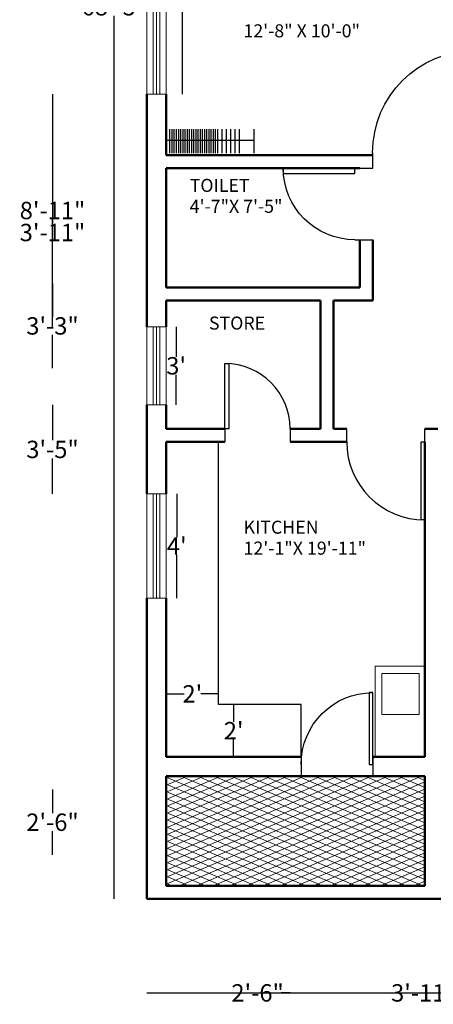
# Model space of a CAD drawing. Units: inches. Extents: x -135167 to -134597, y 156853 to 157819.
# Tile 1 of 5: x -135161 to -134971, y 156853 to 157306. Entities that reach past the tile are written whole.
import ezdxf

# ---------------------------------------------------------------- set-up
doc = ezdxf.new("R2010")
doc.units = ezdxf.units.IN
doc.header["$MEASUREMENT"] = 0
for name, color, linetype, lineweight in [('A-ANNO-DIMS', 4, 'Continuous', 18), ('A-AREA-IDEN', 76, 'Continuous', 25), ('A-FLOR-CASE', 1, 'Continuous', 25), ('A-FLOR-FIXT', 3, 'Continuous', 20), ('A-FLOR-PATT', 8, 'Continuous', 13), ('doors', 5, 'Continuous', 25), ('walls', 2, 'Continuous', 50), ('window', 6, 'Continuous', 18)]:
    doc.layers.add(name, color=color, linetype=linetype, lineweight=lineweight)
doc.styles.get("Standard").update_dxf_attribs({"font": 'arial.ttf'})
doc.dimstyles.get("Standard").update_dxf_attribs({"dimtxt": 8, "dimasz": 0.18, "dimexe": 0.18, "dimexo": 0.0625, "dimgap": 0.09, "dimtad": 0, "dimtih": 1, "dimtoh": 1, "dimdec": 0, "dimzin": 0, "dimdsep": 46, "dimlunit": 3, "dimtxsty": 'Standard', "dimblk": 'ARCHTICK', "dimcen": 0.09, "dimse1": 1, "dimse2": 1, "dimadec": 0, "dimazin": 0, "dimtfac": 1, "dimtdec": 0, "dimtofl": 0, "dimtmove": 0, "dimatfit": 3, "dimldrblk": 'DOTSMALL', "dimfxl": 1, "dimtolj": 1, "dimtzin": 0, "dimarcsym": 0})

# ---------------------------------------------------------------- blocks, each defined once
blk = doc.blocks.new('*U13')
for p, q in [((0, 0), (0, -6)), ((30, 0), (30, -6))]:
    blk.add_line(p, q)
blk.add_lwpolyline([(0, 0), (0, 30), (1.75, 30), (1.75, 0)], close=True)
blk.add_arc((0, 0), 30, 0, 90)
blk = doc.blocks.new('*U6')
for p, q in [((0, 0), (0, -6)), ((40, 0), (40, -6))]:
    blk.add_line(p, q)
blk.add_lwpolyline([(0, 0), (0, 40), (1.75, 40), (1.75, 0)], close=True)
blk.add_arc((0, 0), 40, 0, 90)
blk = doc.blocks.new('*U12')
for p, q in [((0, 0), (0, -6)), ((24, 0), (24, -6))]:
    blk.add_line(p, q)
blk.add_lwpolyline([(0, 0), (0, 24), (1.75, 24), (1.75, 0)], close=True)
blk.add_arc((0, 0), 24, 0, 90)
blk = doc.blocks.new('*U14')
for p, q in [((0, 0), (0, -6)), ((36, 0), (36, -6))]:
    blk.add_line(p, q)
blk.add_lwpolyline([(0, 0), (0, 36), (1.75, 36), (1.75, 0)], close=True)
blk.add_arc((0, 0), 36, 0, 90)
blk = doc.blocks.new('*U9')
for p, q in [((-36, 0), (-36, 6)), ((0, 0), (0, 6))]:
    blk.add_line(p, q)
blk.add_lwpolyline([(0, 0), (0, -36), (-1.75, -36), (-1.75, 0)], close=True)
blk.add_arc((0, 0), 36, 180, 270)
blk = doc.blocks.new('_ArchTick')
at = {"color": 0, "linetype": 'ByBlock', "const_width": 0.15}
blk.add_lwpolyline([(-0.5, -0.5), (0.5, 0.5)], dxfattribs=at)
blk = doc.blocks.new('*D20')
at = {"layer": 'A-ANNO-DIMS', "color": 0, "lineweight": -2, "transparency": 16777216}
for p, q in [((-135117.79, 157722.94), (-135117.79, 157316.42)), ((-135117.79, 156901.55), (-135117.79, 157308.07))]:
    blk.add_line(p, q, dxfattribs=at)
at = {"layer": 'Defpoints', "color": 0, "transparency": 16777216}
for p in [(-135117.79, 157722.94), (-135102.89, 157722.94), (-135102.89, 156901.55)]:
    blk.add_point(p, dxfattribs=at)
at = {"layer": 'A-ANNO-DIMS', "color": 0, "lineweight": -2, "transparency": 16777216, "xscale": 0.18, "yscale": 0.18, "zscale": 0.18}
for p, rotation in [((-135117.79, 157722.94), 90), ((-135117.79, 156901.55), 270)]:
    blk.add_blockref('_ArchTick', p, dxfattribs=dict(at, rotation=rotation))
at = {"layer": 'A-ANNO-DIMS', "color": 0, "transparency": 16777216, "insert": (-135117.79, 157312.25), "char_height": 8, "attachment_point": 5}
blk.add_mtext('\\A1;68\'-5"', dxfattribs=at)
blk = doc.blocks.new('_DotSmall')
at = {"color": 0, "linetype": 'ByBlock', "const_width": 0.5}
blk.add_lwpolyline([(-0.0625, 0, 1), (0.0625, 0, 1)], format="xyb", close=True, dxfattribs=at)
blk = doc.blocks.new('*D33')
at = {"layer": 'A-ANNO-DIMS', "color": 0, "lineweight": -2, "transparency": 16777216}
for p, q in [((-135086.43, 157367.94), (-135086.43, 157324.12)), ((-135086.43, 157271.94), (-135086.43, 157315.77))]:
    blk.add_line(p, q, dxfattribs=at)
at = {"layer": 'Defpoints', "color": 0, "transparency": 16777216}
for p in [(-135093.89, 157367.94), (-135086.43, 157367.94), (-135093.89, 157271.94)]:
    blk.add_point(p, dxfattribs=at)
at = {"layer": 'A-ANNO-DIMS', "color": 0, "lineweight": -2, "transparency": 16777216, "xscale": 0.18, "yscale": 0.18, "zscale": 0.18}
for p, rotation in [((-135086.43, 157367.94), 90), ((-135086.43, 157271.94), 270)]:
    blk.add_blockref('_ArchTick', p, dxfattribs=dict(at, rotation=rotation))
at = {"layer": 'A-ANNO-DIMS', "color": 0, "transparency": 16777216, "insert": (-135086.43, 157319.94), "char_height": 8, "attachment_point": 5}
blk.add_mtext("\\A1;8'", dxfattribs=at)
blk = doc.blocks.new('*D34')
at = {"layer": 'A-ANNO-DIMS', "color": 0, "lineweight": -2, "transparency": 16777216}
for p, q in [((-135089.35, 157164.94), (-135089.35, 157151.12)), ((-135089.35, 157128.94), (-135089.35, 157142.77))]:
    blk.add_line(p, q, dxfattribs=at)
at = {"layer": 'Defpoints', "color": 0, "transparency": 16777216}
for p in [(-135093.89, 157164.94), (-135089.35, 157164.94), (-135093.89, 157128.94)]:
    blk.add_point(p, dxfattribs=at)
at = {"layer": 'A-ANNO-DIMS', "color": 0, "lineweight": -2, "transparency": 16777216, "xscale": 0.18, "yscale": 0.18, "zscale": 0.18}
for p, rotation in [((-135089.35, 157164.94), 90), ((-135089.35, 157128.94), 270)]:
    blk.add_blockref('_ArchTick', p, dxfattribs=dict(at, rotation=rotation))
at = {"layer": 'A-ANNO-DIMS', "color": 0, "transparency": 16777216, "insert": (-135089.35, 157146.94), "char_height": 8, "attachment_point": 5}
blk.add_mtext("\\A1;3'", dxfattribs=at)
blk = doc.blocks.new('*D35')
at = {"layer": 'A-ANNO-DIMS', "color": 0, "lineweight": -2, "transparency": 16777216}
for p, q in [((-135089.08, 157087.94), (-135089.08, 157068.03)), ((-135089.08, 157039.94), (-135089.08, 157059.85))]:
    blk.add_line(p, q, dxfattribs=at)
at = {"layer": 'Defpoints', "color": 0, "transparency": 16777216}
for p in [(-135093.89, 157087.94), (-135089.08, 157087.94), (-135093.89, 157039.94)]:
    blk.add_point(p, dxfattribs=at)
at = {"layer": 'A-ANNO-DIMS', "color": 0, "lineweight": -2, "transparency": 16777216, "xscale": 0.18, "yscale": 0.18, "zscale": 0.18}
for p, rotation in [((-135089.08, 157087.94), 90), ((-135089.08, 157039.94), 270)]:
    blk.add_blockref('_ArchTick', p, dxfattribs=dict(at, rotation=rotation))
at = {"layer": 'A-ANNO-DIMS', "color": 0, "transparency": 16777216, "insert": (-135089.08, 157063.94), "char_height": 8, "attachment_point": 5}
blk.add_mtext("\\A1;4'", dxfattribs=at)
blk = doc.blocks.new('*D36')
at = {"layer": 'A-ANNO-DIMS', "color": 0, "lineweight": -2, "transparency": 16777216}
for p, q in [((-135062.9, 156990.94), (-135062.9, 156983.05)), ((-135062.9, 156966.94), (-135062.9, 156974.84))]:
    blk.add_line(p, q, dxfattribs=at)
at = {"layer": 'Defpoints', "color": 0, "transparency": 16777216}
for p in [(-135060.63, 156990.94), (-135062.9, 156966.94), (-135061.48, 156966.94)]:
    blk.add_point(p, dxfattribs=at)
at = {"layer": 'A-ANNO-DIMS', "color": 0, "lineweight": -2, "transparency": 16777216, "xscale": 0.18, "yscale": 0.18, "zscale": 0.18}
for p, rotation in [((-135062.9, 156990.94), 90), ((-135062.9, 156966.94), 270)]:
    blk.add_blockref('_ArchTick', p, dxfattribs=dict(at, rotation=rotation))
at = {"layer": 'A-ANNO-DIMS', "color": 0, "transparency": 16777216, "insert": (-135062.9, 156978.94), "char_height": 8, "attachment_point": 5}
blk.add_mtext("\\A1;2'", dxfattribs=at)
blk = doc.blocks.new('*D37')
at = {"layer": 'A-ANNO-DIMS', "color": 0, "lineweight": -2, "transparency": 16777216}
for p, q in [((-135093.89, 156995.88), (-135085.72, 156995.88)), ((-135069.89, 156995.88), (-135078.05, 156995.88))]:
    blk.add_line(p, q, dxfattribs=at)
at = {"layer": 'Defpoints', "color": 0, "transparency": 16777216}
for p in [(-135093.89, 156995.88), (-135093.89, 156990.94), (-135069.89, 156990.94)]:
    blk.add_point(p, dxfattribs=at)
at = {"layer": 'A-ANNO-DIMS', "color": 0, "lineweight": -2, "transparency": 16777216, "xscale": 0.18, "yscale": 0.18, "zscale": 0.18, "rotation": 180}
blk.add_blockref('_ArchTick', (-135093.89, 156995.88), dxfattribs=at)
at = {"layer": 'A-ANNO-DIMS', "color": 0, "lineweight": -2, "transparency": 16777216, "xscale": 0.18, "yscale": 0.18, "zscale": 0.18}
blk.add_blockref('_ArchTick', (-135069.89, 156995.88), dxfattribs=at)
at = {"layer": 'A-ANNO-DIMS', "color": 0, "transparency": 16777216, "insert": (-135081.89, 156995.88), "char_height": 8, "attachment_point": 5}
blk.add_mtext("\\A1;2'", dxfattribs=at)
blk = doc.blocks.new('WIN-36IN')
for p, q in [((0, 0), (0, 9)), ((0, 9), (36, 9)), ((0, 6), (36, 6)), ((36, 0), (36, 9)), ((0, 4.5), (36, 4.5)), ((0, 3), (36, 3)), ((0, 0), (36, 0))]:
    blk.add_line(p, q)
blk = doc.blocks.new('WIN-96IN')
for p, q in [((0, 96), (9, 96)), ((0, 96), (0, 0)), ((3, 96), (3, 0)), ((4.5, 96), (4.5, 0)), ((6, 96), (6, 0)), ((9, 96), (9, 0)), ((0, 0), (9, 0))]:
    blk.add_line(p, q)
blk = doc.blocks.new('WIN-48IN')
for p, q in [((0, 48), (9, 48)), ((0, 0), (0, 48)), ((3, 0), (3, 48)), ((4.5, 0), (4.5, 48)), ((6, 0), (6, 48)), ((9, 0), (9, 48)), ((0, 0), (9, 0))]:
    blk.add_line(p, q)
blk = doc.blocks.new('*D54')
at = {"layer": 'A-ANNO-DIMS', "color": 0, "lineweight": -2, "transparency": 16777216}
for p, q in [((-135102.89, 156858.2), (-134897.21, 156858.2)), ((-134663.89, 156858.2), (-134869.56, 156858.2))]:
    blk.add_line(p, q, dxfattribs=at)
at = {"layer": 'Defpoints', "color": 0, "transparency": 16777216}
for p in [(-134663.89, 157136.8), (-135102.89, 156901.55), (-134663.89, 156858.2)]:
    blk.add_point(p, dxfattribs=at)
at = {"layer": 'A-ANNO-DIMS', "color": 0, "lineweight": -2, "transparency": 16777216, "xscale": 0.18, "yscale": 0.18, "zscale": 0.18, "rotation": 180}
blk.add_blockref('_ArchTick', (-135102.89, 156858.2), dxfattribs=at)
at = {"layer": 'A-ANNO-DIMS', "color": 0, "lineweight": -2, "transparency": 16777216, "xscale": 0.18, "yscale": 0.18, "zscale": 0.18}
blk.add_blockref('_ArchTick', (-134663.89, 156858.2), dxfattribs=at)
at = {"layer": 'A-ANNO-DIMS', "color": 0, "transparency": 16777216, "insert": (-134883.39, 156858.2), "char_height": 8, "attachment_point": 5}
blk.add_mtext('\\A1;36\'-7"', dxfattribs=at)
blk = doc.blocks.new('*D59')
at = {"layer": 'A-ANNO-DIMS', "color": 0, "lineweight": -2, "transparency": 16777216}
for p, q in [((-135146.24, 157271.94), (-135146.24, 157222.62)), ((-135146.24, 157164.94), (-135146.24, 157214.27))]:
    blk.add_line(p, q, dxfattribs=at)
at = {"layer": 'Defpoints', "color": 0, "transparency": 16777216}
for p in [(-135102.89, 157271.94), (-135146.24, 157164.94), (-135102.89, 157164.94)]:
    blk.add_point(p, dxfattribs=at)
at = {"layer": 'A-ANNO-DIMS', "color": 0, "lineweight": -2, "transparency": 16777216, "xscale": 0.18, "yscale": 0.18, "zscale": 0.18}
for p, rotation in [((-135146.24, 157271.94), 90), ((-135146.24, 157164.94), 270)]:
    blk.add_blockref('_ArchTick', p, dxfattribs=dict(at, rotation=rotation))
at = {"layer": 'A-ANNO-DIMS', "color": 0, "transparency": 16777216, "insert": (-135146.24, 157218.44), "char_height": 8, "attachment_point": 5}
blk.add_mtext('\\A1;8\'-11"', dxfattribs=at)
blk = doc.blocks.new('*D60')
at = {"layer": 'A-ANNO-DIMS', "color": 0, "lineweight": -2, "transparency": 16777216}
for p, q in [((-135146.24, 157128.94), (-135146.24, 157112.62)), ((-135146.24, 157087.94), (-135146.24, 157104.27))]:
    blk.add_line(p, q, dxfattribs=at)
at = {"layer": 'Defpoints', "color": 0, "transparency": 16777216}
for p in [(-135102.89, 157128.94), (-135146.24, 157087.94), (-135102.89, 157087.94)]:
    blk.add_point(p, dxfattribs=at)
at = {"layer": 'A-ANNO-DIMS', "color": 0, "lineweight": -2, "transparency": 16777216, "xscale": 0.18, "yscale": 0.18, "zscale": 0.18}
for p, rotation in [((-135146.24, 157128.94), 90), ((-135146.24, 157087.94), 270)]:
    blk.add_blockref('_ArchTick', p, dxfattribs=dict(at, rotation=rotation))
at = {"layer": 'A-ANNO-DIMS', "color": 0, "transparency": 16777216, "insert": (-135146.24, 157108.44), "char_height": 8, "attachment_point": 5}
blk.add_mtext('\\A1;3\'-5"', dxfattribs=at)
blk = doc.blocks.new('*D79')
at = {"layer": 'A-ANNO-DIMS', "color": 0, "lineweight": -2, "transparency": 16777216}
for p, q in [((-135146.24, 157231.8), (-135146.24, 157212.48)), ((-135146.24, 157184.8), (-135146.24, 157204.12))]:
    blk.add_line(p, q, dxfattribs=at)
at = {"layer": 'Defpoints', "color": 0, "transparency": 16777216}
for p in [(-135146.24, 157231.8), (-134753.89, 157231.8), (-134753.89, 157184.8)]:
    blk.add_point(p, dxfattribs=at)
at = {"layer": 'A-ANNO-DIMS', "color": 0, "lineweight": -2, "transparency": 16777216, "xscale": 0.18, "yscale": 0.18, "zscale": 0.18}
for p, rotation in [((-135146.24, 157231.8), 90), ((-135146.24, 157184.8), 270)]:
    blk.add_blockref('_ArchTick', p, dxfattribs=dict(at, rotation=rotation))
at = {"layer": 'A-ANNO-DIMS', "color": 0, "transparency": 16777216, "insert": (-135146.24, 157208.3), "char_height": 8, "attachment_point": 5}
blk.add_mtext('\\A1;3\'-11"', dxfattribs=at)
blk = doc.blocks.new('*D80')
at = {"layer": 'A-ANNO-DIMS', "color": 0, "lineweight": -2, "transparency": 16777216}
for p, q in [((-135146.24, 157184.8), (-135146.24, 157169.48)), ((-135146.24, 157145.8), (-135146.24, 157161.12))]:
    blk.add_line(p, q, dxfattribs=at)
at = {"layer": 'Defpoints', "color": 0, "transparency": 16777216}
for p in [(-135146.24, 157184.8), (-134753.89, 157184.8), (-134753.89, 157145.8)]:
    blk.add_point(p, dxfattribs=at)
at = {"layer": 'A-ANNO-DIMS', "color": 0, "lineweight": -2, "transparency": 16777216, "xscale": 0.18, "yscale": 0.18, "zscale": 0.18}
for p, rotation in [((-135146.24, 157184.8), 90), ((-135146.24, 157145.8), 270)]:
    blk.add_blockref('_ArchTick', p, dxfattribs=dict(at, rotation=rotation))
at = {"layer": 'A-ANNO-DIMS', "color": 0, "transparency": 16777216, "insert": (-135146.24, 157165.3), "char_height": 8, "attachment_point": 5}
blk.add_mtext('\\A1;3\'-3"', dxfattribs=at)
blk = doc.blocks.new('*D84')
at = {"layer": 'A-ANNO-DIMS', "color": 0, "lineweight": -2, "transparency": 16777216}
for p, q in [((-134998.89, 156858.2), (-134989.21, 156858.2)), ((-134951.89, 156858.2), (-134961.56, 156858.2))]:
    blk.add_line(p, q, dxfattribs=at)
at = {"layer": 'Defpoints', "color": 0, "transparency": 16777216}
for p in [(-134998.89, 157237.94), (-134951.89, 157237.94), (-134951.89, 156858.2)]:
    blk.add_point(p, dxfattribs=at)
at = {"layer": 'A-ANNO-DIMS', "color": 0, "lineweight": -2, "transparency": 16777216, "xscale": 0.18, "yscale": 0.18, "zscale": 0.18, "rotation": 180}
blk.add_blockref('_ArchTick', (-134998.89, 156858.2), dxfattribs=at)
at = {"layer": 'A-ANNO-DIMS', "color": 0, "lineweight": -2, "transparency": 16777216, "xscale": 0.18, "yscale": 0.18, "zscale": 0.18}
blk.add_blockref('_ArchTick', (-134951.89, 156858.2), dxfattribs=at)
at = {"layer": 'A-ANNO-DIMS', "color": 0, "transparency": 16777216, "insert": (-134975.39, 156858.2), "char_height": 8, "attachment_point": 5}
blk.add_mtext('\\A1;3\'-11"', dxfattribs=at)
blk = doc.blocks.new('*D85')
at = {"layer": 'A-ANNO-DIMS', "color": 0, "lineweight": -2, "transparency": 16777216}
for p, q in [((-134620.54, 157237.94), (-134620.54, 157225.62)), ((-134620.54, 157204.94), (-134620.54, 157217.27))]:
    blk.add_line(p, q, dxfattribs=at)
at = {"layer": 'Defpoints', "color": 0, "transparency": 16777216}
for p in [(-135004.89, 157237.94), (-135004.89, 157204.94), (-134620.54, 157204.94)]:
    blk.add_point(p, dxfattribs=at)
at = {"layer": 'A-ANNO-DIMS', "color": 0, "lineweight": -2, "transparency": 16777216, "xscale": 0.18, "yscale": 0.18, "zscale": 0.18}
for p, rotation in [((-134620.54, 157237.94), 90), ((-134620.54, 157204.94), 270)]:
    blk.add_blockref('_ArchTick', p, dxfattribs=dict(at, rotation=rotation))
at = {"layer": 'A-ANNO-DIMS', "color": 0, "transparency": 16777216, "insert": (-134620.54, 157221.44), "char_height": 8, "attachment_point": 5}
blk.add_mtext('\\A1;2\'-9"', dxfattribs=at)
blk = doc.blocks.new('*D86')
at = {"layer": 'A-ANNO-DIMS', "color": 0, "lineweight": -2, "transparency": 16777216}
for p, q in [((-135010.89, 157806.8), (-135003.61, 157806.8)), ((-134974.89, 157806.8), (-134982.17, 157806.8))]:
    blk.add_line(p, q, dxfattribs=at)
at = {"layer": 'Defpoints', "color": 0, "transparency": 16777216}
for p in [(-134974.89, 157806.8), (-135010.89, 157117.94), (-134974.89, 157117.94)]:
    blk.add_point(p, dxfattribs=at)
at = {"layer": 'A-ANNO-DIMS', "color": 0, "lineweight": -2, "transparency": 16777216, "xscale": 0.18, "yscale": 0.18, "zscale": 0.18, "rotation": 180}
blk.add_blockref('_ArchTick', (-135010.89, 157806.8), dxfattribs=at)
at = {"layer": 'A-ANNO-DIMS', "color": 0, "lineweight": -2, "transparency": 16777216, "xscale": 0.18, "yscale": 0.18, "zscale": 0.18}
blk.add_blockref('_ArchTick', (-134974.89, 157806.8), dxfattribs=at)
at = {"layer": 'A-ANNO-DIMS', "color": 0, "transparency": 16777216, "insert": (-134992.89, 157806.8), "char_height": 8, "attachment_point": 5}
blk.add_mtext('\\A1;3\'-0"', dxfattribs=at)
blk = doc.blocks.new('*D87')
at = {"layer": 'A-ANNO-DIMS', "color": 0, "lineweight": -2, "transparency": 16777216}
for p, q in [((-135066.89, 156858.2), (-135062.68, 156858.2)), ((-135036.89, 156858.2), (-135041.09, 156858.2))]:
    blk.add_line(p, q, dxfattribs=at)
at = {"layer": 'Defpoints', "color": 0, "transparency": 16777216}
for p in [(-135066.89, 157111.94), (-135036.89, 157111.94), (-135036.89, 156858.2)]:
    blk.add_point(p, dxfattribs=at)
at = {"layer": 'A-ANNO-DIMS', "color": 0, "lineweight": -2, "transparency": 16777216, "xscale": 0.18, "yscale": 0.18, "zscale": 0.18, "rotation": 180}
blk.add_blockref('_ArchTick', (-135066.89, 156858.2), dxfattribs=at)
at = {"layer": 'A-ANNO-DIMS', "color": 0, "lineweight": -2, "transparency": 16777216, "xscale": 0.18, "yscale": 0.18, "zscale": 0.18}
blk.add_blockref('_ArchTick', (-135036.89, 156858.2), dxfattribs=at)
at = {"layer": 'A-ANNO-DIMS', "color": 0, "transparency": 16777216, "insert": (-135051.89, 156858.2), "char_height": 8, "attachment_point": 5}
blk.add_mtext('\\A1;2\'-6"', dxfattribs=at)
blk = doc.blocks.new('*D88')
at = {"layer": 'A-ANNO-DIMS', "color": 0, "lineweight": -2, "transparency": 16777216}
for p, q in [((-135031.89, 157806.8), (-135026.18, 157806.8)), ((-134998.89, 157806.8), (-135004.59, 157806.8))]:
    blk.add_line(p, q, dxfattribs=at)
at = {"layer": 'Defpoints', "color": 0, "transparency": 16777216}
for p in [(-134998.89, 157806.8), (-135031.89, 156966.94), (-134998.89, 156966.94)]:
    blk.add_point(p, dxfattribs=at)
at = {"layer": 'A-ANNO-DIMS', "color": 0, "lineweight": -2, "transparency": 16777216, "xscale": 0.18, "yscale": 0.18, "zscale": 0.18, "rotation": 180}
blk.add_blockref('_ArchTick', (-135031.89, 157806.8), dxfattribs=at)
at = {"layer": 'A-ANNO-DIMS', "color": 0, "lineweight": -2, "transparency": 16777216, "xscale": 0.18, "yscale": 0.18, "zscale": 0.18}
blk.add_blockref('_ArchTick', (-134998.89, 157806.8), dxfattribs=at)
at = {"layer": 'A-ANNO-DIMS', "color": 0, "transparency": 16777216, "insert": (-135015.39, 157806.8), "char_height": 8, "attachment_point": 5}
blk.add_mtext('\\A1;2\'-9"', dxfattribs=at)
blk = doc.blocks.new('*D91')
at = {"layer": 'A-ANNO-DIMS', "color": 0, "lineweight": -2, "transparency": 16777216}
for p, q in [((-135146.24, 156951.78), (-135146.24, 156940.95)), ((-135146.24, 156921.78), (-135146.24, 156932.6))]:
    blk.add_line(p, q, dxfattribs=at)
at = {"layer": 'Defpoints', "color": 0, "transparency": 16777216}
for p in [(-134797.39, 156951.78), (-135146.24, 156921.78), (-134797.39, 156921.78)]:
    blk.add_point(p, dxfattribs=at)
at = {"layer": 'A-ANNO-DIMS', "color": 0, "lineweight": -2, "transparency": 16777216, "xscale": 0.18, "yscale": 0.18, "zscale": 0.18}
for p, rotation in [((-135146.24, 156951.78), 90), ((-135146.24, 156921.78), 270)]:
    blk.add_blockref('_ArchTick', p, dxfattribs=dict(at, rotation=rotation))
at = {"layer": 'A-ANNO-DIMS', "color": 0, "transparency": 16777216, "insert": (-135146.24, 156936.78), "char_height": 8, "attachment_point": 5}
blk.add_mtext('\\A1;2\'-6"', dxfattribs=at)
blk = doc.blocks.new('*D92')
at = {"layer": 'A-ANNO-DIMS', "color": 0, "lineweight": -2, "transparency": 16777216}
for p, q in [((-134987.89, 156858.2), (-134955.58, 156858.2)), ((-134901.89, 156858.2), (-134934.2, 156858.2))]:
    blk.add_line(p, q, dxfattribs=at)
at = {"layer": 'Defpoints', "color": 0, "transparency": 16777216}
for p in [(-134987.89, 157647.94), (-134901.89, 157647.94), (-134901.89, 156858.2)]:
    blk.add_point(p, dxfattribs=at)
at = {"layer": 'A-ANNO-DIMS', "color": 0, "lineweight": -2, "transparency": 16777216, "xscale": 0.18, "yscale": 0.18, "zscale": 0.18, "rotation": 180}
blk.add_blockref('_ArchTick', (-134987.89, 156858.2), dxfattribs=at)
at = {"layer": 'A-ANNO-DIMS', "color": 0, "lineweight": -2, "transparency": 16777216, "xscale": 0.18, "yscale": 0.18, "zscale": 0.18}
blk.add_blockref('_ArchTick', (-134901.89, 156858.2), dxfattribs=at)
at = {"layer": 'A-ANNO-DIMS', "color": 0, "transparency": 16777216, "insert": (-134944.89, 156858.2), "char_height": 8, "attachment_point": 5}
blk.add_mtext('\\A1;7\'-2"', dxfattribs=at)

msp = doc.modelspace()

# ---------------------------------------------------------------- hatches: boundary and pattern name
at = {"layer": 'A-FLOR-PATT'}
h = msp.add_hatch(dxfattribs=at)
h.set_pattern_fill('ANSI31', color=256, scale=24, angle=-22.049143, style=0)
h.paths.add_polyline_path([(-135093.89, 156907.55), (-134974.89, 156907.55), (-134974.89, 156957.94), (-135093.89, 156957.94)])
h = msp.add_hatch(dxfattribs=at)
h.set_pattern_fill('ANSI31', color=256, scale=24, angle=112.049143, style=0)
h.paths.add_polyline_path([(-135093.89, 156907.55), (-134974.89, 156907.55), (-134974.89, 156957.94), (-135093.89, 156957.94)])

# ---------------------------------------------------------------- linework, layer by layer
at = {"layer": 'A-FLOR-CASE'}
for p, q in [((-135092.34, 157255.95), (-135092.34, 157244.82)), ((-135091.34, 157255.95), (-135091.34, 157244.82)), ((-135090.34, 157255.95), (-135090.34, 157244.82)), ((-135089.34, 157255.95), (-135089.34, 157244.82)), ((-135088.34, 157255.95), (-135088.34, 157244.82)), ((-135087.34, 157255.95), (-135087.34, 157244.82)), ((-135086.34, 157255.95), (-135086.34, 157244.82)), ((-135085.34, 157255.95), (-135085.34, 157244.82)), ((-135084.34, 157255.95), (-135084.34, 157244.82)), ((-135083.34, 157255.95), (-135083.34, 157244.82)), ((-135082.34, 157255.95), (-135082.34, 157244.82)), ((-135081.34, 157255.95), (-135081.34, 157244.82)), ((-135080.34, 157255.95), (-135080.34, 157244.82)), ((-135079.34, 157255.95), (-135079.34, 157244.82)), ((-135078.34, 157255.95), (-135078.34, 157244.82)), ((-135077.34, 157255.95), (-135077.34, 157244.82)), ((-135076.34, 157255.95), (-135076.34, 157244.82)), ((-135075.34, 157255.95), (-135075.34, 157244.82)), ((-135074.34, 157255.95), (-135074.34, 157244.82)), ((-135073.34, 157255.95), (-135073.34, 157244.82)), ((-135072.34, 157255.95), (-135072.34, 157244.82)), ((-135071.34, 157255.95), (-135071.34, 157244.82)), ((-135070.34, 157255.95), (-135070.34, 157244.82)), ((-135068.34, 157255.95), (-135068.34, 157244.82)), ((-135066.34, 157255.95), (-135066.34, 157244.82)), ((-135064.34, 157255.95), (-135064.34, 157244.82)), ((-135062.34, 157255.95), (-135062.34, 157244.82)), ((-135062.34, 157255.95), (-135062.34, 157244.82)), ((-135060.34, 157255.95), (-135060.34, 157244.82)), ((-135053.65, 157255.95), (-135053.65, 157244.82)), ((-135053.65, 157250.6), (-135093.89, 157250.6)), ((-135069.89, 156990.94), (-135069.89, 157111.94)), ((-135031.89, 156990.94), (-135069.89, 156990.94)), ((-135031.89, 156966.94), (-135031.89, 156990.94))]:
    msp.add_line(p, q, dxfattribs=at)
at = {"layer": 'A-FLOR-FIXT'}
for points in [[(-134974.89, 156966.94), (-134997.84, 156966.94), (-134997.84, 157008.71), (-134974.89, 157008.71)], [(-134994.65, 157005.23), (-134977.54, 157005.23), (-134977.54, 156986.41), (-134994.65, 156986.41)]]:
    msp.add_lwpolyline(points, close=True, dxfattribs=at)
at = {"layer": 'doors'}
for p, q in [((-134998.89, 157237.94), (-134998.89, 157243.94)), ((-135004.89, 157237.94), (-134998.89, 157237.94)), ((-135004.89, 157204.94), (-134998.89, 157204.94)), ((-135066.89, 157117.94), (-135066.89, 157111.94)), ((-135036.89, 157117.94), (-135036.89, 157111.94)), ((-135010.89, 157111.94), (-135010.89, 157117.94)), ((-134974.89, 157111.94), (-134974.89, 157117.94)), ((-135031.89, 156966.94), (-135031.89, 156957.94)), ((-134998.89, 156966.94), (-134998.89, 156957.94))]:
    msp.add_line(p, q, dxfattribs=at)
at = {"layer": 'walls'}
for p, q in [((-135102.89, 157164.94), (-135102.89, 157271.94)), ((-135093.89, 157243.94), (-135093.89, 157271.94)), ((-135093.89, 157243.94), (-134998.89, 157243.94)), ((-135093.89, 157237.94), (-135004.89, 157237.94)), ((-135093.89, 157182.94), (-135093.89, 157237.94)), ((-135004.89, 157182.94), (-135004.89, 157204.94)), ((-134998.89, 157176.94), (-134998.89, 157204.94)), ((-135093.89, 157182.94), (-135004.89, 157182.94)), ((-135093.89, 157176.94), (-135022.89, 157176.94)), ((-135093.89, 157164.94), (-135093.89, 157176.94)), ((-135022.89, 157117.94), (-135022.89, 157176.94)), ((-135016.89, 157117.94), (-135016.89, 157176.94)), ((-135016.89, 157176.94), (-134998.89, 157176.94)), ((-135102.89, 157087.94), (-135102.89, 157128.94)), ((-135093.89, 157117.94), (-135093.89, 157128.94)), ((-135093.89, 157117.94), (-135066.89, 157117.94)), ((-135036.89, 157117.94), (-135022.89, 157117.94)), ((-135016.89, 157117.94), (-135010.89, 157117.94)), ((-134974.89, 157117.94), (-134968.89, 157117.94)), ((-135093.89, 157111.94), (-135066.89, 157111.94)), ((-135093.89, 157087.94), (-135093.89, 157111.94)), ((-135036.89, 157111.94), (-135010.89, 157111.94)), ((-134974.89, 156966.94), (-134974.89, 157111.94)), ((-135102.89, 156901.55), (-135102.89, 157039.94)), ((-135093.89, 156966.94), (-135093.89, 157039.94)), ((-135093.89, 156966.94), (-135031.89, 156966.94)), ((-134998.89, 156966.94), (-134974.89, 156966.94)), ((-135093.89, 156907.55), (-135093.89, 156957.94)), ((-135093.89, 156957.94), (-134998.89, 156957.94)), ((-134998.89, 156957.94), (-134974.89, 156957.94)), ((-134974.89, 156907.55), (-134974.89, 156957.94)), ((-135093.89, 156907.55), (-134974.89, 156907.55)), ((-135102.89, 156901.55), (-134744.89, 156901.55))]:
    msp.add_line(p, q, dxfattribs=at)

# ---------------------------------------------------------------- block references
at = {"layer": 'doors'}
for name, p, xscale, yscale, zscale in [('*U6', (-134951.89, 157245.01), -1.177072109473595, 1.177072109473595, 1.177072109473595), ('*U14', (-134998.89, 156963.44), -0.9168796826214972, 0.9168796826214972, 0.9168796826214972)]:
    msp.add_blockref(name, p, dxfattribs=dict(at, xscale=xscale, yscale=yscale, zscale=zscale))
at = {"layer": 'doors', "xscale": -1.373377664918856, "yscale": 1.373377664918856, "zscale": 1.373377664918856, "rotation": 90}
msp.add_blockref('*U12', (-135007.1, 157237.94), dxfattribs=at)
at = {"layer": 'doors'}
for name, p in [('*U13', (-135066.89, 157117.94)), ('*U9', (-134974.89, 157111.94))]:
    msp.add_blockref(name, p, dxfattribs=at)
at = {"layer": 'window'}
for name, p, rotation in [('WIN-96IN', (-135093.89, 157367.94), 180), ('WIN-36IN', (-135093.89, 157128.94), 90.00000000000003)]:
    msp.add_blockref(name, p, dxfattribs=dict(at, rotation=rotation))
msp.add_blockref('WIN-48IN', (-135102.89, 157039.94), dxfattribs=at)

# ---------------------------------------------------------------- texts
at = {"layer": 'A-AREA-IDEN'}
for s, p in [('12\'-8" X 10\'-0"', (-135058.39, 157298.16)), ('TOILET ', (-135083.12, 157227)), ('4\'-7"X 7\'-5"', (-135083.12, 157217.36)), ('STORE ', (-135074.27, 157163.6)), ('KITCHEN ', (-135058.33, 157069.62)), ('12\'-1"X 19\'-11"', (-135058.33, 157059.98))]:
    msp.add_text(s, height=6, dxfattribs=at).set_placement(p)

# ---------------------------------------------------------------- dimensions: what is measured, and where the dimension line sits
at = {"layer": 'A-ANNO-DIMS'}
for base, p1, p2, override, picture, middle in [((-134998.89, 157806.8), (-135031.89, 156966.94), (-134998.89, 156966.94), {"dimdec": 1, "dimlfac": 1, "dimrnd": 0, "dimzin": 1, "dimdsep": 46, "dimlunit": 4, "dimfrac": 2}, '*D88', (-135015.39, 157806.8)), ((-134974.89, 157806.8), (-135010.89, 157117.94), (-134974.89, 157117.94), {"dimdec": 1, "dimlfac": 1, "dimrnd": 0, "dimzin": 1, "dimdsep": 46, "dimlunit": 4, "dimfrac": 2}, '*D86', (-134992.89, 157806.8)), ((-134901.89, 156858.2), (-134987.89, 157647.94), (-134901.89, 157647.94), {"dimdec": 1, "dimlfac": 1, "dimrnd": 0, "dimzin": 1, "dimdsep": 46, "dimlunit": 4, "dimfrac": 2}, '*D92', (-134944.89, 156858.2)), ((-134951.89, 156858.2), (-134998.89, 157237.94), (-134951.89, 157237.94), {"dimdec": 1, "dimlfac": 1, "dimrnd": 0, "dimzin": 1, "dimdsep": 46, "dimlunit": 4, "dimfrac": 2}, '*D84', (-134975.39, 156858.2)), ((-134663.89, 156858.2), (-135102.89, 156901.55), (-134663.89, 157136.8), {"dimdec": 1, "dimlfac": 1, "dimrnd": 0, "dimzin": 1, "dimdsep": 46, "dimlunit": 4, "dimfrac": 2}, '*D54', (-134883.39, 156858.2)), ((-135036.89, 156858.2), (-135066.89, 157111.94), (-135036.89, 157111.94), {"dimdec": 1, "dimlfac": 1, "dimrnd": 0, "dimzin": 1, "dimdsep": 46, "dimlunit": 4, "dimfrac": 2}, '*D87', (-135051.89, 156858.2)), ((-135093.89, 156995.88), (-135069.89, 156990.94), (-135093.89, 156990.94), {"dimclrd": 0, "dimclre": 0, "dimclrt": 0}, '*D37', (-135081.89, 156995.88))]:
    dim = msp.add_linear_dim(base=base, p1=p1, p2=p2, dimstyle='Standard', override=override, dxfattribs=at)
    dim.commit()
    dim.dimension.update_dxf_attribs({"geometry": picture, "text_midpoint": middle})
for base, p1, p2, override, picture, middle in [((-135117.79, 157722.94), (-135102.89, 156901.55), (-135102.89, 157722.94), {"dimclrd": 0, "dimclre": 0, "dimclrt": 0}, '*D20', (-135117.79, 157312.25)), ((-135086.43, 157367.94), (-135093.89, 157271.94), (-135093.89, 157367.94), {"dimclrd": 0, "dimclre": 0, "dimclrt": 0}, '*D33', (-135086.43, 157319.94)), ((-135146.24, 157164.94), (-135102.89, 157271.94), (-135102.89, 157164.94), {"dimdec": 1, "dimlfac": 1, "dimrnd": 0, "dimzin": 1, "dimdsep": 46, "dimlunit": 4, "dimfrac": 2}, '*D59', (-135146.24, 157218.44)), ((-134620.54, 157204.94), (-135004.89, 157237.94), (-135004.89, 157204.94), {"dimdec": 1, "dimlfac": 1, "dimrnd": 0, "dimzin": 1, "dimdsep": 46, "dimlunit": 4, "dimfrac": 2}, '*D85', (-134620.54, 157221.44)), ((-135146.24, 157231.8), (-134753.89, 157184.8), (-134753.89, 157231.8), {"dimdec": 1, "dimlfac": 1, "dimrnd": 0, "dimzin": 1, "dimdsep": 46, "dimlunit": 4, "dimfrac": 2}, '*D79', (-135146.24, 157208.3)), ((-135146.24, 157184.8), (-134753.89, 157145.8), (-134753.89, 157184.8), {"dimdec": 1, "dimlfac": 1, "dimrnd": 0, "dimzin": 1, "dimdsep": 46, "dimlunit": 4, "dimfrac": 2}, '*D80', (-135146.24, 157165.3)), ((-135089.35, 157164.94), (-135093.89, 157128.94), (-135093.89, 157164.94), {"dimclrd": 0, "dimclre": 0, "dimclrt": 0}, '*D34', (-135089.35, 157146.94)), ((-135146.24, 157087.94), (-135102.89, 157128.94), (-135102.89, 157087.94), {"dimdec": 1, "dimlfac": 1, "dimrnd": 0, "dimzin": 1, "dimdsep": 46, "dimlunit": 4, "dimfrac": 2}, '*D60', (-135146.24, 157108.44)), ((-135089.08, 157087.94), (-135093.89, 157039.94), (-135093.89, 157087.94), {"dimclrd": 0, "dimclre": 0, "dimclrt": 0}, '*D35', (-135089.08, 157063.94)), ((-135062.9, 156966.94), (-135060.63, 156990.94), (-135061.48, 156966.94), {"dimclrd": 0, "dimclre": 0, "dimclrt": 0}, '*D36', (-135062.9, 156978.94)), ((-135146.24, 156921.78), (-134797.39, 156951.78), (-134797.39, 156921.78), {"dimdec": 1, "dimlfac": 1, "dimrnd": 0, "dimzin": 1, "dimdsep": 46, "dimlunit": 4, "dimfrac": 2}, '*D91', (-135146.24, 156936.78))]:
    dim = msp.add_linear_dim(base=base, p1=p1, p2=p2, angle=90, dimstyle='Standard', override=override, dxfattribs=at)
    dim.commit()
    dim.dimension.update_dxf_attribs({"geometry": picture, "text_midpoint": middle})

doc.saveas('drawing.dxf')
